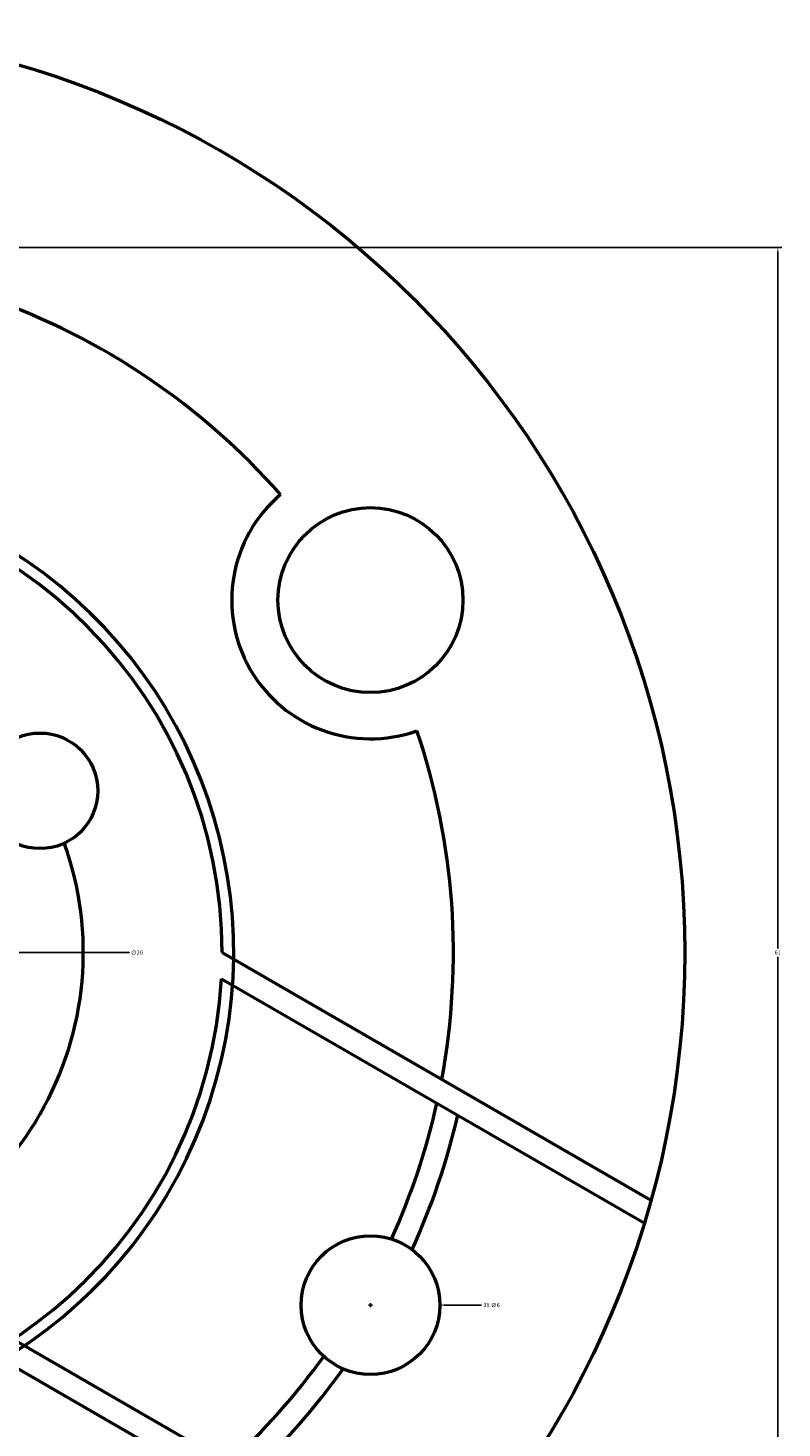
# Model space of a CAD drawing. Units: inches. Extents: x -19.9 to 72.3, y -39.8 to 57.5.
# Tile 8 of 8: x 39.7 to 72.3, y -7.2 to 53.3. Entities that reach past the tile are written whole.
import ezdxf

# ---------------------------------------------------------------- set-up
doc = ezdxf.new("R2010")
doc.units = ezdxf.units.IN
doc.header["$MEASUREMENT"] = 0
for name, color, linetype, lineweight in [('M-DIMS', 2, 'Continuous', 18), ('M-OUTL', 7, 'Continuous', 50), ('M-OUTL-HOLE', 7, 'Continuous', 50), ('M-OUTL-SLOT', 7, 'Continuous', 50)]:
    doc.layers.add(name, color=color, linetype=linetype, lineweight=lineweight)
doc.styles.get("Standard").update_dxf_attribs({"font": 'arial.ttf'})
doc.dimstyles.get("Standard").update_dxf_attribs({"dimtxt": 0.18, "dimasz": 0.18, "dimexe": 0.18, "dimexo": 0.0625, "dimgap": 0.09, "dimtad": 0, "dimtih": 1, "dimtoh": 1, "dimdec": 4, "dimzin": 0, "dimdsep": 46, "dimtxsty": 'Standard', "dimcen": 0.09, "dimadec": 0, "dimazin": 0, "dimtfac": 1, "dimtdec": 4, "dimtofl": 0, "dimtmove": 0, "dimatfit": 3, "dimfxl": 1, "dimtolj": 1, "dimtzin": 0, "dimarcsym": 0})

# ---------------------------------------------------------------- blocks, each defined once
blk = doc.blocks.new('FLANGE-MOUNT-D8-RELIEVED')
blk.add_circle((0, 0), 4)
for centre, radius, start, end in [((26.414, -15.25), 30, 109.47122, 138.65617), ((0, 0), 6, 250.42865, 49.57135), ((26.414, -15.25), 30, 161.34383, 190.52878)]:
    blk.add_arc(centre, radius, start, end)
blk = doc.blocks.new('FLANGE-HOLE-D6')
blk.add_circle((0, 0), 3)
blk = doc.blocks.new('HUB-HOLE-D5')
blk.add_circle((0, 0), 2.5)
blk = doc.blocks.new('FLANGE-STRAIGHT-SLOT')
for p, q in [((0, 0), (0, 21.114)), ((1, -0.54), (1, 20.869))]:
    blk.add_line(p, q)
blk = doc.blocks.new('FLANGE-INTERRUPTED-ARC-SLOT')
for radius, start, end in [(30, 192.5424, 204.39482), (31, 193.12273, 204.48604), (30, 215.60518, 227.4576), (31, 215.51396, 226.87727)]:
    blk.add_arc((26.414, 15.25), radius, start, end)
blk = doc.blocks.new('*D6')
at = {"layer": 'Defpoints', "color": 0, "transparency": 16777216}
for p in [(28.06, 43.841), (28.06, -17.159), (72.086, -17.159)]:
    blk.add_point(p, dxfattribs=at)
at = {"layer": 'M-DIMS', "color": 0, "lineweight": -2, "transparency": 16777216}
for p, q in [((28.122, 43.841), (72.266, 43.841)), ((72.086, 43.661), (72.086, 13.523)), ((72.086, -16.979), (72.086, 13.159)), ((28.122, -17.159), (72.266, -17.159))]:
    blk.add_line(p, q, dxfattribs=at)
at = {"layer": 'M-DIMS', "color": 0, "transparency": 16777216}
for points in [[(72.056, 43.661), (72.116, 43.661), (72.086, 43.841)], [(72.056, -16.979), (72.116, -16.979), (72.086, -17.159)]]:
    blk.add_solid(points, dxfattribs=at)
at = {"layer": 'M-DIMS', "color": 0, "transparency": 16777216, "insert": (72.086, 13.341), "char_height": 0.18, "attachment_point": 5}
blk.add_mtext('\\A1;61', dxfattribs=at)
blk = doc.blocks.new('*D11')
at = {"layer": 'Defpoints', "color": 0, "transparency": 16777216}
for p in [(5.703, 46.51), (50.417, -19.828)]:
    blk.add_point(p, dxfattribs=at)
at = {"layer": 'M-DIMS', "color": 0, "lineweight": -2, "transparency": 16777216}
for p, q in [((27.97, 13.341), (28.15, 13.341)), ((28.06, 13.251), (28.06, 13.431)), ((63.831, -39.729), (50.517, -19.977)), ((64.011, -39.729), (63.831, -39.729))]:
    blk.add_line(p, q, dxfattribs=at)
at = {"layer": 'M-DIMS', "color": 0, "transparency": 16777216}
blk.add_solid([(50.542, -19.96), (50.492, -19.994), (50.417, -19.828)], dxfattribs=at)
at = {"layer": 'M-DIMS', "color": 0, "transparency": 16777216, "insert": (64.327, -39.729), "char_height": 0.18, "attachment_point": 5}
blk.add_mtext('\\A1;∅80', dxfattribs=at)
blk = doc.blocks.new('*D18')
at = {"layer": 'Defpoints', "color": 0, "transparency": 16777216}
for p in [(18.06, 13.342), (38.06, 13.341)]:
    blk.add_point(p, dxfattribs=at)
at = {"layer": 'M-DIMS', "color": 0, "lineweight": -2, "transparency": 16777216}
for p, q in [((27.97, 13.341), (28.15, 13.341)), ((28.06, 13.251), (28.06, 13.431)), ((44.06, 13.341), (38.24, 13.341))]:
    blk.add_line(p, q, dxfattribs=at)
at = {"layer": 'M-DIMS', "color": 0, "transparency": 16777216}
blk.add_solid([(38.24, 13.371), (38.24, 13.311), (38.06, 13.341)], dxfattribs=at)
at = {"layer": 'M-DIMS', "color": 0, "transparency": 16777216, "insert": (44.376, 13.341), "char_height": 0.18, "attachment_point": 5}
blk.add_mtext('\\A1;∅20', dxfattribs=at)
blk = doc.blocks.new('*D21')
at = {"layer": 'Defpoints', "color": 0, "transparency": 16777216}
for p in [(51.474, -1.908), (57.474, -1.909)]:
    blk.add_point(p, dxfattribs=at)
at = {"layer": 'M-DIMS', "color": 0, "lineweight": -2, "transparency": 16777216}
for p, q in [((54.384, -1.909), (54.564, -1.909)), ((54.474, -1.999), (54.474, -1.819)), ((59.274, -1.909), (57.654, -1.909))]:
    blk.add_line(p, q, dxfattribs=at)
at = {"layer": 'M-DIMS', "color": 0, "transparency": 16777216}
blk.add_solid([(57.654, -1.879), (57.654, -1.939), (57.474, -1.909)], dxfattribs=at)
at = {"layer": 'M-DIMS', "color": 0, "transparency": 16777216, "insert": (59.709, -1.909), "char_height": 0.18, "attachment_point": 5}
blk.add_mtext('\\A1;3X ∅6', dxfattribs=at)

msp = doc.modelspace()

# ---------------------------------------------------------------- linework, layer by layer
at = {"layer": 'M-OUTL'}
msp.add_circle((28.06, 13.341), 40, dxfattribs=at)
for radius, start, end in [(20, 0, 356.74368), (20.5, 183.95835, 60.8036), (14, 280.24503, 19.75497)]:
    msp.add_arc((28.06, 13.341), radius, start, end, dxfattribs=at)

# ---------------------------------------------------------------- block references
at = {"layer": 'M-OUTL-HOLE'}
for p, rotation in [((54.474, 28.591), 240), ((28.06, -17.159), 120)]:
    msp.add_blockref('FLANGE-MOUNT-D8-RELIEVED', p, dxfattribs=dict(at, rotation=rotation))
for name, p in [('HUB-HOLE-D5', (40.184, 20.341)), ('FLANGE-HOLE-D6', (54.474, -1.909))]:
    msp.add_blockref(name, p, dxfattribs=at)
at = {"layer": 'M-OUTL-SLOT', "extrusion": (0, 0, -1), "zscale": -1, "rotation": 119.9999999999999}
msp.add_blockref('FLANGE-STRAIGHT-SLOT', (-48.028, 12.205), dxfattribs=at)
at = {"layer": 'M-OUTL-SLOT'}
for name, p, rotation in [('FLANGE-INTERRUPTED-ARC-SLOT', (54.474, -1.909), 120), ('FLANGE-STRAIGHT-SLOT', (39.028, -3.383), 240)]:
    msp.add_blockref(name, p, dxfattribs=dict(at, rotation=rotation))

# ---------------------------------------------------------------- dimensions: what is measured, and where the dimension line sits
at = {"layer": 'M-DIMS'}
for p1, p2, picture, middle in [((5.703, 46.51), (50.417, -19.828), '*D11', (64.327, -39.729)), ((18.06, 13.342), (38.06, 13.341), '*D18', (44.06, 13.341))]:
    dim = msp.add_diameter_dim_2p(p1=p1, p2=p2, dimstyle='Standard', override={"dimdec": 0, "dimlfac": 1, "dimrnd": 0, "dimzin": 0, "dimdsep": 46, "dimlunit": 2}, dxfattribs=at)
    dim.commit()
    dim.dimension.update_dxf_attribs({"geometry": picture, "text_midpoint": middle, "dimtype": 163})
dim = msp.add_linear_dim(base=(72.086, -17.159), p1=(28.06, 43.841), p2=(28.06, -17.159), angle=90, dimstyle='Standard', override={"dimdec": 0, "dimlfac": 1, "dimrnd": 0, "dimzin": 0, "dimdsep": 46, "dimlunit": 2}, dxfattribs=at)
dim.commit()
dim.dimension.update_dxf_attribs({"geometry": '*D6', "text_midpoint": (72.086, 13.341)})
dim = msp.add_diameter_dim_2p(p1=(51.474, -1.908), p2=(57.474, -1.909), text='3X <>', dimstyle='Standard', override={"dimdec": 0, "dimlfac": 1, "dimrnd": 0, "dimzin": 0, "dimdsep": 46, "dimlunit": 2}, dxfattribs=at)
dim.commit()
dim.dimension.update_dxf_attribs({"geometry": '*D21', "text_midpoint": (59.274, -1.909), "dimtype": 163})

doc.saveas('drawing.dxf')
